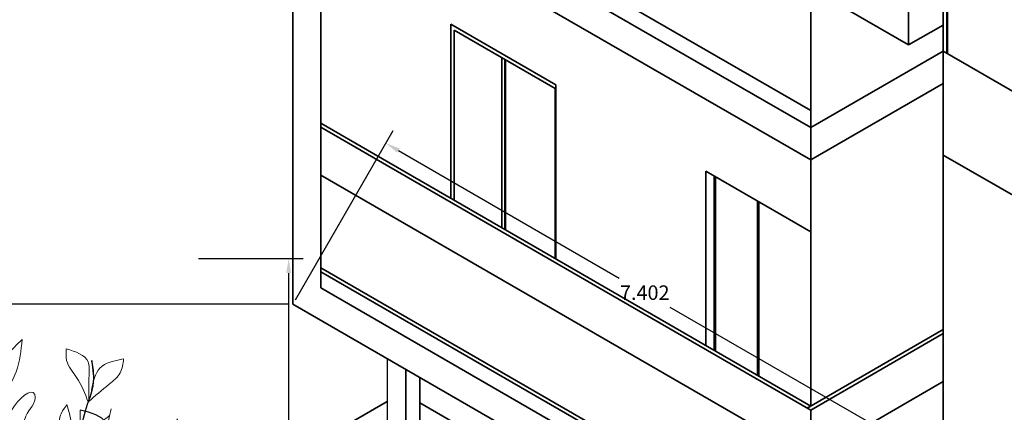
# Model space of a CAD drawing. Units: metres. Extents: x 12735 to 25554, y 20954 to 41989.
# Tile 7 of 15: x 12743.95 to 12756.13, y 20974.68 to 20979.54. Entities that reach past the tile are written whole.
import ezdxf

# ---------------------------------------------------------------- set-up
doc = ezdxf.new("R2010")
doc.units = ezdxf.units.M
doc.layers.get('Defpoints').update_dxf_attribs({"lineweight": 13})
for name, color, linetype, lineweight in [('A-ANNO-DIMS', 2, 'Continuous', 18), ('A-ELEV', 7, 'Continuous', 35), ('C-SITE', 8, 'Continuous', 25), ('TREES', 72, 'Continuous', 18)]:
    doc.layers.add(name, color=color, linetype=linetype, lineweight=lineweight)
doc.layers.add('STEM', color=32, linetype='Continuous')
doc.styles.get("Standard").update_dxf_attribs({"font": 'arial.ttf'})
doc.dimstyles.get("Standard").update_dxf_attribs({"dimtxt": 0.18, "dimasz": 0.18, "dimexe": 0.18, "dimexo": 0.0625, "dimgap": 0.09, "dimtad": 0, "dimtih": 1, "dimtoh": 1, "dimdec": 4, "dimzin": 0, "dimdsep": 46, "dimtxsty": 'Standard', "dimcen": 0.09, "dimadec": 0, "dimazin": 0, "dimtfac": 1, "dimtdec": 4, "dimtofl": 0, "dimtmove": 0, "dimatfit": 3, "dimfxl": 1, "dimtolj": 1, "dimtzin": 0, "dimarcsym": 0})

# ---------------------------------------------------------------- blocks, each defined once
blk = doc.blocks.new('TREES')
blk.add_line((12743.7, 20972.648), (12743.7, 20972.648))
at = {"layer": 'STEM'}
for points, knots in [([(12743.791, 20972.546), (12743.793, 20972.564), (12743.795, 20972.582), (12743.797, 20972.6), (12743.801, 20972.637), (12743.806, 20972.674), (12743.81, 20972.711), (12743.845, 20973.018), (12743.938, 20973.826), (12743.743, 20974.806), (12743.607, 20975.634), (12743.413, 20975.893), (12743.333, 20975.999)], [-0.164913, -0.164913, -0.164913, -0.164913, -0.110972, -0.110972, -0.110972, 0, 0, 0, 0.920963, 2.426088, 2.990404, 3.384799, 3.384799, 3.384799, 3.384799]), ([(12743.7, 20972.648), (12743.691, 20972.807), (12743.671, 20973.194), (12743.257, 20973.699), (12743.111, 20974.379), (12743.038, 20974.998), (12742.993, 20975.377), (12742.974, 20975.54)], [0, 0, 0, 0, 0.469346, 1.137622, 1.869488, 2.521439, 3.013071, 3.013071, 3.013071, 3.013071]), ([(12743.874, 20972.227), (12743.898, 20972.277), (12743.921, 20972.328), (12743.945, 20972.378), (12744.022, 20972.541), (12744.105, 20972.717), (12744.205, 20972.963), (12744.312, 20973.088), (12744.183, 20973.501), (12744.667, 20973.973), (12744.707, 20974.64), (12744.896, 20975.012), (12744.823, 20975.434), (12744.85, 20975.23), (12744.867, 20975.1)], [-0.166951, -0.166951, -0.166951, -0.166951, 0, 0, 0, 0.539768, 0.582066, 0.798222, 0.98781, 1.7696, 2.524754, 2.899414, 3.105113, 3.460848, 3.460848, 3.460848, 3.460848]), ([(12743.728, 20972.218), (12743.63, 20972.372), (12743.383, 20972.76), (12742.753, 20973.07), (12742.291, 20973.419), (12741.984, 20973.759), (12741.959, 20974.098), (12741.675, 20974.346), (12741.563, 20974.543), (12741.494, 20974.663)], [0, 0, 0, 0, 0.542161, 1.359078, 2.03444, 2.290187, 2.703676, 2.968549, 3.382864, 3.382864, 3.382864, 3.382864]), ([(12743.967, 20971.294), (12743.987, 20971.335), (12744.006, 20971.376), (12744.026, 20971.417), (12744.057, 20971.483), (12744.088, 20971.549), (12744.119, 20971.615), (12744.196, 20971.778), (12744.279, 20971.954), (12744.378, 20972.2), (12744.486, 20972.325), (12744.357, 20972.738), (12744.836, 20973.215), (12744.895, 20973.862), (12745.051, 20974.269), (12745.045, 20974.62), (12744.834, 20974.67), (12744.7, 20974.701)], [-0.355099, -0.355099, -0.355099, -0.355099, -0.218492, -0.218492, -0.218492, 0, 0, 0, 0.539768, 0.582066, 0.798222, 0.98781, 1.7696, 2.524754, 2.899414, 3.105113, 3.460848, 3.460848, 3.460848, 3.460848]), ([(12744.175, 20971.633), (12744.383, 20971.767), (12744.692, 20971.967), (12745.149, 20972.305), (12745.828, 20972.463), (12745.606, 20973.185), (12745.967, 20973.583), (12745.99, 20973.882), (12746.002, 20974.029)], [0, 0, 0, 0, 0.736164, 1.094646, 1.754618, 2.392389, 2.840214, 3.27091, 3.27091, 3.27091, 3.27091]), ([(12743.381, 20973.588), (12743.52, 20973.4), (12743.728, 20973.118), (12743.725, 20972.776), (12743.724, 20972.661), (12743.724, 20972.661), (12743.724, 20972.661), (12743.724, 20972.661), (12743.724, 20972.65), (12743.724, 20972.639), (12743.724, 20972.627)], [0, 0, 0, 0, 0.673099, 1.009429, 1.009429, 1.009429, 1.009429, 1.009429, 1.009429, 1.043412, 1.043412, 1.043412, 1.043412]), ([(12743.814, 20972.505), (12743.817, 20972.531), (12743.819, 20972.556), (12743.822, 20972.581), (12743.827, 20972.63), (12743.832, 20972.679), (12743.838, 20972.727), (12743.847, 20972.813), (12743.865, 20972.982), (12743.864, 20973.152), (12743.864, 20973.236)], [-0.2227932, -0.2227932, -0.2227932, -0.2227932, -0.1464713, -0.1464713, -0.1464713, 0, 0, 0, 0.2578951, 0.5103882, 0.5103882, 0.5103882, 0.5103882]), ([(12743.902, 20971.717), (12743.93, 20971.754), (12743.959, 20971.791), (12743.988, 20971.829), (12743.988, 20971.829), (12743.988, 20971.829), (12743.988, 20971.829), (12744.096, 20971.973), (12744.236, 20972.16), (12744.082, 20972.476), (12744.347, 20972.598), (12744.368, 20972.766), (12744.376, 20972.837)], [-0.129757, -0.129757, -0.129757, -0.129757, 0, 0, 0, 0, 0, 0, 0.485118, 0.62751, 0.913144, 1.120766, 1.120766, 1.120766, 1.120766]), ([(12744.111, 20968.725), (12743.967, 20969.837), (12743.799, 20971.142), (12743.712, 20972.453), (12743.7, 20972.648)], [0, 0, 0, 0, 3.359203, 3.944548, 3.944548, 3.944548, 3.944548]), ([(12744.332, 20968.825), (12744.189, 20969.936), (12743.871, 20971.161), (12743.872, 20972.51), (12743.7, 20972.648)], [0, 0, 0, 0, 3.359203, 3.972384, 3.972384, 3.972384, 3.972384]), ([(12743.597, 20972.418), (12743.533, 20972.41), (12743.292, 20972.379), (12742.889, 20972.351), (12742.364, 20972.241), (12741.803, 20972.489), (12741.157, 20972.302), (12740.698, 20972.258), (12740.474, 20972.237)], [0, 0, 0, 0, 0.193148, 0.727923, 1.218416, 1.762371, 2.471743, 3.152626, 3.152626, 3.152626, 3.152626]), ([(12743.181, 20972.372), (12743.296, 20972.37), (12743.441, 20972.368), (12743.583, 20972.39), (12743.613, 20972.395)], [0, 0, 0, 0, 0.3435042, 0.4329772, 0.4329772, 0.4329772, 0.4329772]), ([(12743.948, 20971.264), (12743.975, 20971.305), (12744.002, 20971.345), (12744.029, 20971.386), (12744.029, 20971.386), (12744.029, 20971.386), (12744.029, 20971.386), (12744.129, 20971.55), (12744.289, 20971.812), (12744.368, 20972.107), (12744.398, 20972.218)], [-0.148605, -0.148605, -0.148605, -0.148605, 0, 0, 0, 0, 0, 0, 0.572176, 0.914425, 0.914425, 0.914425, 0.914425]), ([(12743.901, 20971.729), (12743.929, 20971.768), (12743.958, 20971.808), (12743.986, 20971.847), (12743.986, 20971.847), (12743.986, 20971.847), (12743.986, 20971.847), (12744.02, 20971.892), (12744.062, 20971.951), (12744.099, 20972.014), (12744.107, 20972.028)], [-0.1467707, -0.1467707, -0.1467707, -0.1467707, 0, 0, 0, 0, 0, 0, 0.1684242, 0.2179474, 0.2179474, 0.2179474, 0.2179474]), ([(12743.81, 20971.258), (12743.646, 20971.316), (12743.283, 20971.443), (12742.486, 20971.453), (12741.888, 20971.61), (12741.494, 20971.714)], [0, 0, 0, 0, 0.519056, 1.146346, 2.366016, 2.366016, 2.366016, 2.366016])]:
    blk.add_open_spline(points, degree=3, knots=knots, dxfattribs=at)
blk.add_open_spline([(12744.644, 20971.941), (12744.672, 20971.961), (12744.701, 20971.98), (12744.73, 20972)], degree=3, dxfattribs=at)
at = {"layer": 'TREES'}
for points, knots in [([(12743.584, 20975.586), (12743.37, 20975.718), (12743.075, 20975.9), (12743.022, 20976.725), (12743.333, 20976.097), (12743.574, 20975.612)], [0, 0, 0, 0, 0.724771, 1.002271, 1.932196, 1.932196, 1.932196, 1.932196]), ([(12743.021, 20975.14), (12742.985, 20975.224), (12742.928, 20975.356), (12742.766, 20975.539), (12742.854, 20975.638), (12742.901, 20975.69)], [0, 0, 0, 0, 0.2845416, 0.4465287, 0.6279758, 0.6279758, 0.6279758, 0.6279758]), ([(12743.021, 20975.14), (12743.019, 20975.277), (12743.016, 20975.483), (12742.921, 20975.662), (12742.889, 20975.721)], [0, 0, 0, 0, 0.4023849, 0.6031293, 0.6031293, 0.6031293, 0.6031293]), ([(12743.718, 20974.979), (12743.671, 20975.164), (12743.598, 20975.454), (12743.323, 20975.534), (12743.223, 20975.563)], [0, 0, 0, 0, 0.519429, 0.8155501, 0.8155501, 0.8155501, 0.8155501]), ([(12743.223, 20975.563), (12743.266, 20975.448), (12743.36, 20975.195), (12743.592, 20975.055), (12743.718, 20974.979)], [0, 0, 0, 0, 0.3595778, 0.7860105, 0.7860105, 0.7860105, 0.7860105]), ([(12743.737, 20974.871), (12743.729, 20975.055), (12743.718, 20975.333), (12743.914, 20975.516), (12743.981, 20975.578)], [0, 0, 0, 0, 0.5134638, 0.7779111, 0.7779111, 0.7779111, 0.7779111]), ([(12743.737, 20974.871), (12743.801, 20974.971), (12743.939, 20975.186), (12743.966, 20975.441), (12743.981, 20975.578)], [0, 0, 0, 0, 0.351068, 0.7565079, 0.7565079, 0.7565079, 0.7565079]), ([(12741.648, 20974.411), (12741.519, 20974.547), (12741.281, 20974.798), (12741.642, 20974.995), (12741.673, 20975.511), (12741.684, 20975.149), (12741.787, 20975.033), (12741.768, 20974.824), (12741.781, 20974.575), (12741.641, 20974.411), (12741.569, 20974.326)], [0, 0, 0, 0, 0.446457, 0.821839, 1.096823, 1.294203, 1.491123, 1.594729, 1.894892, 2.216107, 2.216107, 2.216107, 2.216107]), ([(12743.031, 20975.058), (12743.048, 20975.139), (12743.077, 20975.281), (12743.184, 20975.377), (12743.231, 20975.418)], [0, 0, 0, 0, 0.2398723, 0.4207027, 0.4207027, 0.4207027, 0.4207027]), ([(12743.037, 20975.007), (12743.075, 20975.058), (12743.166, 20975.181), (12743.207, 20975.33), (12743.231, 20975.418)], [0, 0, 0, 0, 0.1895117, 0.457602, 0.457602, 0.457602, 0.457602]), ([(12744.796, 20974.806), (12744.757, 20974.909), (12744.688, 20975.088), (12744.514, 20975.28), (12744.523, 20975.414), (12744.526, 20975.464)], [0, 0, 0, 0, 0.3323117, 0.5782809, 0.7232611, 0.7232611, 0.7232611, 0.7232611]), ([(12744.805, 20974.813), (12744.804, 20974.918), (12744.803, 20975.076), (12744.822, 20975.37), (12744.643, 20975.427), (12744.526, 20975.464)], [0, 0, 0, 0, 0.3224266, 0.4885617, 0.8037384, 0.8037384, 0.8037384, 0.8037384]), ([(12743.07, 20974.733), (12742.98, 20974.863), (12742.848, 20975.053), (12742.433, 20975.446), (12742.649, 20974.915), (12742.651, 20974.573), (12742.961, 20974.576), (12743.034, 20974.678), (12743.071, 20974.73)], [0, 0, 0, 0, 0.54832, 0.799685, 1.166614, 1.565159, 1.742127, 1.925713, 1.925713, 1.925713, 1.925713]), ([(12744.796, 20974.806), (12744.882, 20974.878), (12745.017, 20974.992), (12745.211, 20975.15), (12745.228, 20975.277), (12745.236, 20975.337)], [0, 0, 0, 0, 0.3416822, 0.5370609, 0.7122352, 0.7122352, 0.7122352, 0.7122352]), ([(12744.839, 20974.951), (12744.859, 20975.055), (12744.903, 20975.272), (12745.122, 20975.315), (12745.236, 20975.337)], [0, 0, 0, 0, 0.2913456, 0.6064398, 0.6064398, 0.6064398, 0.6064398]), ([(12743.814, 20974.4), (12743.798, 20974.494), (12743.764, 20974.693), (12744.115, 20975.006), (12744.156, 20974.79), (12744.01, 20974.677), (12743.989, 20974.434), (12743.864, 20974.438), (12743.809, 20974.439)], [0, 0, 0, 0, 0.311146, 0.650746, 0.669061, 0.940573, 1.125337, 1.270427, 1.270427, 1.270427, 1.270427]), ([(12743.191, 20974.047), (12743.14, 20974.139), (12743.026, 20974.346), (12743.367, 20974.877), (12743.354, 20974.597), (12743.309, 20974.413), (12743.358, 20974.125), (12743.218, 20974.059), (12743.191, 20974.047)], [0, 0, 0, 0, 0.337622, 0.758697, 0.837919, 1.040495, 1.406258, 1.489574, 1.489574, 1.489574, 1.489574]), ([(12744.509, 20973.941), (12744.486, 20974.093), (12744.451, 20974.322), (12744.425, 20974.623), (12744.504, 20974.731), (12744.534, 20974.773)], [0, 0, 0, 0, 0.4681587, 0.7056034, 0.8580265, 0.8580265, 0.8580265, 0.8580265]), ([(12744.534, 20974.773), (12744.556, 20974.698), (12744.634, 20974.425), (12744.562, 20974.144), (12744.509, 20973.941)], [0, 0, 0, 0, 0.2327329, 0.8431329, 0.8431329, 0.8431329, 0.8431329]), ([(12742.028, 20973.754), (12742.003, 20973.912), (12741.953, 20974.218), (12742.174, 20974.414), (12742.283, 20974.81), (12742.258, 20974.48), (12742.304, 20974.323), (12742.246, 20974.069), (12742.227, 20973.932), (12742.006, 20973.671), (12742.066, 20973.72), (12742.075, 20973.727)], [0, 0, 0, 0, 0.436736, 0.842969, 1.012738, 1.21393, 1.403734, 1.613178, 1.897283, 2.067562, 2.097274, 2.097274, 2.097274, 2.097274]), ([(12744.554, 20973.975), (12744.669, 20974.016), (12744.893, 20974.094), (12745.019, 20974.421), (12745.06, 20974.624), (12745.08, 20974.72)], [0, 0, 0, 0, 0.348929, 0.678298, 0.9763146, 0.9763146, 0.9763146, 0.9763146]), ([(12744.97, 20974.043), (12744.931, 20974.146), (12744.862, 20974.325), (12744.688, 20974.517), (12744.697, 20974.651), (12744.7, 20974.701)], [0, 0, 0, 0, 0.3323117, 0.5782809, 0.7232611, 0.7232611, 0.7232611, 0.7232611]), ([(12743.835, 20974.249), (12743.789, 20974.346), (12743.724, 20974.484), (12743.556, 20974.594), (12743.468, 20974.601), (12743.424, 20974.604)], [0, 0, 0, 0, 0.3158223, 0.4463774, 0.5774617, 0.5774617, 0.5774617, 0.5774617]), ([(12743.424, 20974.604), (12743.442, 20974.527), (12743.487, 20974.324), (12743.715, 20974.191), (12743.841, 20974.206), (12743.841, 20974.206)], [0, 0, 0, 0, 0.2361186, 0.6165307, 0.6167763, 0.6167763, 0.6167763, 0.6167763]), ([(12744.618, 20974.118), (12744.717, 20974.268), (12744.844, 20974.462), (12745.022, 20974.606), (12745.062, 20974.638)], [0, 0, 0, 0, 0.5333846, 0.686651, 0.686651, 0.686651, 0.686651]), ([(12744.97, 20974.043), (12745.056, 20974.115), (12745.191, 20974.229), (12745.385, 20974.387), (12745.402, 20974.514), (12745.41, 20974.574)], [0, 0, 0, 0, 0.3416822, 0.5370609, 0.7122352, 0.7122352, 0.7122352, 0.7122352]), ([(12745.013, 20974.188), (12745.033, 20974.292), (12745.077, 20974.509), (12745.296, 20974.552), (12745.41, 20974.574)], [0, 0, 0, 0, 0.2913456, 0.6064398, 0.6064398, 0.6064398, 0.6064398]), ([(12745.957, 20973.706), (12745.908, 20973.835), (12745.798, 20974.123), (12745.864, 20974.427), (12745.9, 20974.594)], [0, 0, 0, 0, 0.4051126, 0.906838, 0.906838, 0.906838, 0.906838]), ([(12745.9, 20974.594), (12745.955, 20974.471), (12746.037, 20974.287), (12746.01, 20974.092), (12746.002, 20974.029)], [0, 0, 0, 0, 0.3943838, 0.5836156, 0.5836156, 0.5836156, 0.5836156]), ([(12743.128, 20974.182), (12743.019, 20974.275), (12742.841, 20974.427), (12742.65, 20974.313), (12742.577, 20974.27)], [0, 0, 0, 0, 0.3785086, 0.6144536, 0.6144536, 0.6144536, 0.6144536]), ([(12745.785, 20973.361), (12745.68, 20973.449), (12745.404, 20973.684), (12745.451, 20974.057), (12745.481, 20974.288)], [0, 0, 0, 0, 0.391493, 1.034106, 1.034106, 1.034106, 1.034106]), ([(12745.481, 20974.288), (12745.577, 20974.138), (12745.76, 20973.855), (12745.777, 20973.519), (12745.785, 20973.361)], [0, 0, 0, 0, 0.5245256, 0.9915723, 0.9915723, 0.9915723, 0.9915723]), ([(12741.943, 20974.016), (12741.835, 20974.13), (12741.594, 20974.382), (12741.272, 20973.991), (12740.687, 20974.27), (12741.289, 20973.836), (12741.63, 20973.742), (12741.878, 20973.799), (12742.016, 20973.831)], [0, 0, 0, 0, 0.397812, 0.88569, 1.156328, 1.66735, 1.991498, 2.394837, 2.394837, 2.394837, 2.394837]), ([(12742.577, 20974.27), (12742.635, 20974.174), (12742.755, 20973.977), (12743.187, 20974.003), (12743.173, 20974.131), (12743.172, 20974.137)], [0, 0, 0, 0, 0.3386751, 0.6999446, 0.7185805, 0.7185805, 0.7185805, 0.7185805]), ([(12743.879, 20973.555), (12743.816, 20973.752), (12743.731, 20974.021), (12743.982, 20974.067), (12744.068, 20974.224), (12744.006, 20973.984), (12744.093, 20973.824), (12743.961, 20973.709), (12743.879, 20973.638)], [0, 0, 0, 0, 0.469961, 0.638827, 0.705595, 0.853148, 1.022788, 1.296962, 1.296962, 1.296962, 1.296962]), ([(12744.356, 20973.647), (12744.309, 20973.708), (12744.202, 20973.846), (12744.245, 20974.018), (12744.268, 20974.113)], [0, 0, 0, 0, 0.2209277, 0.4981889, 0.4981889, 0.4981889, 0.4981889]), ([(12744.268, 20974.113), (12744.323, 20974.065), (12744.46, 20973.94), (12744.395, 20973.758), (12744.356, 20973.647)], [0, 0, 0, 0, 0.203616, 0.5174389, 0.5174389, 0.5174389, 0.5174389]), ([(12742.389, 20973.356), (12742.341, 20973.437), (12742.234, 20973.617), (12742.458, 20973.799), (12742.48, 20973.946), (12742.486, 20973.991)], [0, 0, 0, 0, 0.251735, 0.5591808, 0.6938707, 0.6938707, 0.6938707, 0.6938707]), ([(12742.486, 20973.991), (12742.542, 20973.959), (12742.68, 20973.88), (12742.598, 20973.572), (12742.464, 20973.433), (12742.389, 20973.356)], [0, 0, 0, 0, 0.1746142, 0.4385715, 0.7703441, 0.7703441, 0.7703441, 0.7703441]), ([(12743.381, 20973.588), (12743.369, 20973.67), (12743.344, 20973.833), (12743.453, 20973.958), (12743.508, 20974.02)], [0, 0, 0, 0, 0.2360196, 0.4713289, 0.4713289, 0.4713289, 0.4713289]), ([(12743.381, 20973.588), (12743.434, 20973.649), (12743.541, 20973.774), (12743.519, 20973.937), (12743.508, 20974.02)], [0, 0, 0, 0, 0.2309694, 0.4699481, 0.4699481, 0.4699481, 0.4699481]), ([(12744.683, 20973.178), (12744.66, 20973.33), (12744.625, 20973.559), (12744.599, 20973.86), (12744.677, 20973.968), (12744.708, 20974.01)], [0, 0, 0, 0, 0.4681587, 0.7056034, 0.8580265, 0.8580265, 0.8580265, 0.8580265]), ([(12744.708, 20974.01), (12744.73, 20973.935), (12744.807, 20973.662), (12744.735, 20973.381), (12744.683, 20973.178)], [0, 0, 0, 0, 0.2327329, 0.8431329, 0.8431329, 0.8431329, 0.8431329]), ([(12744.728, 20973.213), (12744.843, 20973.253), (12745.067, 20973.331), (12745.193, 20973.658), (12745.234, 20973.861), (12745.254, 20973.957)], [0, 0, 0, 0, 0.348929, 0.678298, 0.9763146, 0.9763146, 0.9763146, 0.9763146]), ([(12743.851, 20973.09), (12743.747, 20973.196), (12743.578, 20973.368), (12743.647, 20973.644), (12743.671, 20973.769), (12743.679, 20973.81)], [0, 0, 0, 0, 0.4076044, 0.6640272, 0.7921335, 0.7921335, 0.7921335, 0.7921335]), ([(12743.679, 20973.81), (12743.708, 20973.778), (12743.776, 20973.703), (12743.798, 20973.443), (12743.829, 20973.238), (12743.851, 20973.09)], [0, 0, 0, 0, 0.125659, 0.2981213, 0.7527794, 0.7527794, 0.7527794, 0.7527794]), ([(12744.792, 20973.355), (12744.891, 20973.505), (12745.018, 20973.699), (12745.196, 20973.843), (12745.236, 20973.876)], [0, 0, 0, 0, 0.5333846, 0.686651, 0.686651, 0.686651, 0.686651]), ([(12742.221, 20973.506), (12741.989, 20973.602), (12741.674, 20973.731), (12741.536, 20973.471), (12741.5, 20973.404)], [0, 0, 0, 0, 0.6060397, 0.8197481, 0.8197481, 0.8197481, 0.8197481]), ([(12743.364, 20973.617), (12743.288, 20973.661), (12743.124, 20973.754), (12742.939, 20973.715), (12742.84, 20973.694)], [0, 0, 0, 0, 0.2535199, 0.5460217, 0.5460217, 0.5460217, 0.5460217]), ([(12742.84, 20973.694), (12742.956, 20973.634), (12743.128, 20973.545), (12743.306, 20973.6), (12743.364, 20973.617)], [0, 0, 0, 0, 0.369417, 0.546183, 0.546183, 0.546183, 0.546183]), ([(12743.253, 20972.784), (12743.147, 20972.854), (12742.919, 20973.005), (12742.8, 20973.728), (12742.973, 20973.491), (12743.022, 20973.422)], [0, 0, 0, 0, 0.420416, 0.90702, 1.103207, 1.103207, 1.103207, 1.103207]), ([(12743.864, 20973.236), (12743.891, 20973.272), (12743.952, 20973.35), (12744.077, 20973.438), (12744.058, 20973.527), (12744.051, 20973.558)], [0, 0, 0, 0, 0.1377377, 0.3031534, 0.3935537, 0.3935537, 0.3935537, 0.3935537]), ([(12743.866, 20973.267), (12743.872, 20973.352), (12743.881, 20973.49), (12744.004, 20973.539), (12744.051, 20973.558)], [0, 0, 0, 0, 0.2295676, 0.3730638, 0.3730638, 0.3730638, 0.3730638]), ([(12744.268, 20973.425), (12744.32, 20973.505), (12744.424, 20973.666), (12744.615, 20973.662), (12744.711, 20973.66)], [0, 0, 0, 0, 0.2669279, 0.5349854, 0.5349854, 0.5349854, 0.5349854]), ([(12744.268, 20973.425), (12744.336, 20973.433), (12744.51, 20973.454), (12744.635, 20973.582), (12744.711, 20973.66)], [0, 0, 0, 0, 0.1990667, 0.5143408, 0.5143408, 0.5143408, 0.5143408]), ([(12741.493, 20973.429), (12741.634, 20973.396), (12741.906, 20973.333), (12742.16, 20973.449), (12742.283, 20973.505)], [0, 0, 0, 0, 0.420024, 0.8136231, 0.8136231, 0.8136231, 0.8136231]), ([(12743.022, 20973.422), (12743.059, 20973.426), (12743.334, 20973.456), (12743.256, 20972.956), (12743.349, 20972.723), (12743.36, 20972.696)], [0, 0, 0, 0, 0.1039343, 0.7792863, 0.8705393, 0.8705393, 0.8705393, 0.8705393]), ([(12745.697, 20972.996), (12745.547, 20972.999), (12745.238, 20973.004), (12745.268, 20973.314), (12745.283, 20973.473)], [0, 0, 0, 0, 0.3799868, 0.779071, 0.779071, 0.779071, 0.779071]), ([(12745.283, 20973.473), (12745.354, 20973.458), (12745.585, 20973.409), (12745.651, 20973.165), (12745.697, 20972.996)], [0, 0, 0, 0, 0.2074949, 0.6743984, 0.6743984, 0.6743984, 0.6743984]), ([(12743.621, 20973.151), (12743.561, 20973.233), (12743.473, 20973.354), (12743.333, 20973.334), (12743.288, 20973.327)], [0, 0, 0, 0, 0.2726158, 0.4022356, 0.4022356, 0.4022356, 0.4022356]), ([(12743.288, 20973.327), (12743.325, 20973.265), (12743.399, 20973.138), (12743.546, 20973.147), (12743.621, 20973.151)], [0, 0, 0, 0, 0.199886, 0.4070645, 0.4070645, 0.4070645, 0.4070645]), ([(12744.53, 20972.884), (12744.482, 20972.945), (12744.376, 20973.084), (12744.419, 20973.255), (12744.442, 20973.351)], [0, 0, 0, 0, 0.2209277, 0.4981889, 0.4981889, 0.4981889, 0.4981889]), ([(12744.442, 20973.351), (12744.496, 20973.302), (12744.634, 20973.177), (12744.569, 20972.995), (12744.53, 20972.884)], [0, 0, 0, 0, 0.203616, 0.5174389, 0.5174389, 0.5174389, 0.5174389]), ([(12741.595, 20972.406), (12741.523, 20972.496), (12741.318, 20972.752), (12741.336, 20973.087), (12741.348, 20973.304)], [0, 0, 0, 0, 0.3390919, 0.9589007, 0.9589007, 0.9589007, 0.9589007]), ([(12741.348, 20973.304), (12741.406, 20973.227), (12741.6, 20972.969), (12741.591, 20972.637), (12741.585, 20972.405)], [0, 0, 0, 0, 0.2865181, 0.9509807, 0.9509807, 0.9509807, 0.9509807]), ([(12745.697, 20972.996), (12745.724, 20973.08), (12745.77, 20973.226), (12745.915, 20973.262), (12745.976, 20973.277)], [0, 0, 0, 0, 0.2439478, 0.4222058, 0.4222058, 0.4222058, 0.4222058]), ([(12745.697, 20972.996), (12745.764, 20973.024), (12745.897, 20973.078), (12745.95, 20973.211), (12745.976, 20973.277)], [0, 0, 0, 0, 0.2073861, 0.4117039, 0.4117039, 0.4117039, 0.4117039]), ([(12743.669, 20972.977), (12743.606, 20973.025), (12743.504, 20973.102), (12743.398, 20973.043), (12743.358, 20973.021)], [0, 0, 0, 0, 0.2119595, 0.340544, 0.340544, 0.340544, 0.340544]), ([(12744.074, 20972.655), (12744.086, 20972.673), (12744.124, 20972.731), (12743.998, 20972.782), (12744.014, 20972.867), (12744.011, 20972.925), (12744.052, 20972.944), (12744.07, 20973.015), (12743.988, 20973.027), (12743.97, 20973.091), (12744.03, 20973.11), (12744.072, 20973.132), (12744.097, 20973.169), (12744.133, 20973.163), (12744.172, 20973.164), (12744.216, 20973.136), (12744.296, 20973.17), (12744.282, 20973.105), (12744.259, 20973.057), (12744.341, 20973.048), (12744.328, 20972.986), (12744.32, 20972.935), (12744.299, 20972.884), (12744.258, 20972.852), (12744.236, 20972.821), (12744.215, 20972.805), (12744.179, 20972.793), (12744.139, 20972.807), (12744.095, 20972.746), (12744.111, 20972.739), (12744.111, 20972.739)], [0, 0, 0, 0, 0.055886, 0.185472, 0.25227, 0.305988, 0.338368, 0.378405, 0.48523, 0.4997, 0.565031, 0.618654, 0.656012, 0.680602, 0.71942, 0.77395, 0.836088, 0.890088, 0.913694, 0.979696, 1.032481, 1.0683, 1.142133, 1.186825, 1.224162, 1.25438, 1.26551, 1.333296, 1.383591, 1.385324, 1.385324, 1.385324, 1.385324]), ([(12742.983, 20972.961), (12742.799, 20973.009), (12742.463, 20973.098), (12742.071, 20972.928), (12741.893, 20972.798), (12741.839, 20972.759)], [0, 0, 0, 0, 0.553894, 1.01265, 1.215779, 1.215779, 1.215779, 1.215779]), ([(12741.839, 20972.759), (12741.949, 20972.7), (12742.323, 20972.501), (12742.684, 20972.786), (12742.939, 20972.987)], [0, 0, 0, 0, 0.355589, 1.206871, 1.206871, 1.206871, 1.206871]), ([(12743.358, 20973.021), (12743.426, 20972.983), (12743.527, 20972.926), (12743.633, 20972.964), (12743.669, 20972.977)], [0, 0, 0, 0, 0.2166399, 0.3265492, 0.3265492, 0.3265492, 0.3265492]), ([(12741.358, 20972.366), (12741.291, 20972.434), (12741.162, 20972.564), (12740.909, 20972.646), (12740.492, 20972.989), (12740.719, 20972.381), (12740.905, 20972.253), (12741.437, 20972.382), (12741.361, 20972.366), (12741.358, 20972.366)], [0, 0, 0, 0, 0.274554, 0.529523, 0.902439, 1.220606, 1.740632, 1.953969, 1.962894, 1.962894, 1.962894, 1.962894]), ([(12742.858, 20972.779), (12743.034, 20972.81), (12743.375, 20972.87), (12743.295, 20972.539), (12743.257, 20972.379)], [0, 0, 0, 0, 0.4156133, 0.8046117, 0.8046117, 0.8046117, 0.8046117]), ([(12744.299, 20972.615), (12744.284, 20972.657), (12744.255, 20972.734), (12744.322, 20972.816), (12744.34, 20972.869), (12744.347, 20972.89)], [0, 0, 0, 0, 0.1248577, 0.2264879, 0.2926557, 0.2926557, 0.2926557, 0.2926557]), ([(12744.442, 20972.662), (12744.494, 20972.743), (12744.598, 20972.903), (12744.789, 20972.899), (12744.885, 20972.897)], [0, 0, 0, 0, 0.2669279, 0.5349854, 0.5349854, 0.5349854, 0.5349854]), ([(12744.442, 20972.662), (12744.51, 20972.671), (12744.684, 20972.691), (12744.809, 20972.819), (12744.885, 20972.897)], [0, 0, 0, 0, 0.1990667, 0.5143408, 0.5143408, 0.5143408, 0.5143408]), ([(12745.557, 20972.46), (12745.505, 20972.545), (12745.415, 20972.69), (12745.509, 20972.826), (12745.548, 20972.882)], [0, 0, 0, 0, 0.2672291, 0.4594629, 0.4594629, 0.4594629, 0.4594629]), ([(12745.548, 20972.882), (12745.623, 20972.785), (12745.735, 20972.639), (12745.619, 20972.519), (12745.581, 20972.479)], [0, 0, 0, 0, 0.3063433, 0.4579535, 0.4579535, 0.4579535, 0.4579535]), ([(12745.681, 20972.634), (12745.776, 20972.643), (12745.97, 20972.661), (12746.056, 20972.838), (12746.1, 20972.929)], [0, 0, 0, 0, 0.2646598, 0.5464061, 0.5464061, 0.5464061, 0.5464061]), ([(12745.691, 20972.679), (12745.723, 20972.743), (12745.803, 20972.904), (12745.989, 20972.919), (12746.1, 20972.929)], [0, 0, 0, 0, 0.2025395, 0.5100625, 0.5100625, 0.5100625, 0.5100625]), ([(12743.257, 20972.379), (12743.071, 20972.409), (12742.794, 20972.453), (12742.842, 20972.698), (12742.858, 20972.779)], [0, 0, 0, 0, 0.4478858, 0.6692237, 0.6692237, 0.6692237, 0.6692237]), ([(12744.14, 20972.455), (12744.129, 20972.498), (12744.112, 20972.571), (12744.173, 20972.643), (12744.195, 20972.684), (12744.204, 20972.7)], [0, 0, 0, 0, 0.124617, 0.2107396, 0.2658134, 0.2658134, 0.2658134, 0.2658134]), ([(12744.14, 20972.455), (12744.155, 20972.485), (12744.181, 20972.535), (12744.225, 20972.615), (12744.212, 20972.669), (12744.204, 20972.7)], [0, 0, 0, 0, 0.1037237, 0.1704768, 0.2630686, 0.2630686, 0.2630686, 0.2630686]), ([(12745.276, 20972.317), (12745.252, 20972.391), (12745.204, 20972.544), (12745.32, 20972.655), (12745.379, 20972.712)], [0, 0, 0, 0, 0.2148949, 0.4418034, 0.4418034, 0.4418034, 0.4418034]), ([(12745.276, 20972.317), (12745.329, 20972.378), (12745.429, 20972.493), (12745.395, 20972.642), (12745.379, 20972.712)], [0, 0, 0, 0, 0.2259484, 0.4304915, 0.4304915, 0.4304915, 0.4304915]), ([(12740.645, 20972.254), (12740.532, 20972.287), (12740.33, 20972.345), (12740.37, 20972.543), (12740.387, 20972.63)], [0, 0, 0, 0, 0.300298, 0.5327787, 0.5327787, 0.5327787, 0.5327787]), ([(12740.387, 20972.63), (12740.446, 20972.602), (12740.598, 20972.53), (12740.627, 20972.359), (12740.645, 20972.254)], [0, 0, 0, 0, 0.1847401, 0.4807235, 0.4807235, 0.4807235, 0.4807235]), ([(12742.916, 20972.343), (12742.772, 20972.452), (12742.448, 20972.697), (12742.076, 20972.511), (12741.869, 20972.407)], [0, 0, 0, 0, 0.501704, 1.133573, 1.133573, 1.133573, 1.133573]), ([(12744.192, 20972.515), (12744.244, 20972.502), (12744.335, 20972.479), (12744.372, 20972.56), (12744.387, 20972.593)], [0, 0, 0, 0, 0.1401829, 0.239855, 0.239855, 0.239855, 0.239855]), ([(12744.25, 20972.55), (12744.272, 20972.566), (12744.314, 20972.595), (12744.364, 20972.594), (12744.387, 20972.593)], [0, 0, 0, 0, 0.0790636, 0.1468534, 0.1468534, 0.1468534, 0.1468534]), ([(12744.137, 20972.378), (12744.147, 20972.414), (12744.168, 20972.49), (12744.249, 20972.485), (12744.292, 20972.483)], [0, 0, 0, 0, 0.0982704, 0.2114853, 0.2114853, 0.2114853, 0.2114853]), ([(12744.137, 20972.378), (12744.171, 20972.382), (12744.241, 20972.388), (12744.274, 20972.45), (12744.292, 20972.483)], [0, 0, 0, 0, 0.0955829, 0.1975677, 0.1975677, 0.1975677, 0.1975677]), ([(12744.868, 20972.097), (12744.937, 20972.148), (12745.072, 20972.246), (12745.072, 20972.413), (12745.073, 20972.494)], [0, 0, 0, 0, 0.2403434, 0.4714363, 0.4714363, 0.4714363, 0.4714363]), ([(12744.868, 20972.097), (12744.895, 20972.212), (12744.931, 20972.363), (12745.046, 20972.458), (12745.074, 20972.481)], [0, 0, 0, 0, 0.3374321, 0.4432568, 0.4432568, 0.4432568, 0.4432568]), ([(12745.582, 20972.481), (12745.667, 20972.516), (12745.814, 20972.576), (12745.958, 20972.516), (12746.019, 20972.491)], [0, 0, 0, 0, 0.2625898, 0.453199, 0.453199, 0.453199, 0.453199]), ([(12745.582, 20972.481), (12745.658, 20972.433), (12745.808, 20972.341), (12745.95, 20972.442), (12746.019, 20972.491)], [0, 0, 0, 0, 0.2451587, 0.4783488, 0.4783488, 0.4783488, 0.4783488]), ([(12741.223, 20971.823), (12741.319, 20971.881), (12741.571, 20972.033), (12741.755, 20972.264), (12741.869, 20972.407)], [0, 0, 0, 0, 0.3340001, 0.876507, 0.876507, 0.876507, 0.876507]), ([(12741.595, 20972.406), (12741.515, 20972.319), (12741.356, 20972.147), (12741.267, 20971.93), (12741.223, 20971.823)], [0, 0, 0, 0, 0.3521388, 0.6963584, 0.6963584, 0.6963584, 0.6963584]), ([(12743.181, 20972.372), (12743.094, 20972.305), (12742.907, 20972.162), (12742.991, 20971.938), (12743.035, 20971.819)], [0, 0, 0, 0, 0.2977969, 0.6372286, 0.6372286, 0.6372286, 0.6372286]), ([(12743.035, 20971.819), (12743.147, 20971.88), (12743.383, 20972.009), (12743.25, 20972.247), (12743.181, 20972.372)], [0, 0, 0, 0, 0.3275492, 0.688496, 0.688496, 0.688496, 0.688496]), ([(12744.145, 20972.348), (12744.132, 20972.384), (12744.105, 20972.455), (12744.032, 20972.434), (12743.996, 20972.423)], [0, 0, 0, 0, 0.098996, 0.196743, 0.196743, 0.196743, 0.196743]), ([(12743.996, 20972.423), (12744.027, 20972.377), (12744.069, 20972.315), (12744.13, 20972.341), (12744.146, 20972.347)], [0, 0, 0, 0, 0.1368513, 0.185287, 0.185287, 0.185287, 0.185287]), ([(12745.422, 20972.381), (12745.493, 20972.379), (12745.657, 20972.373), (12745.791, 20972.276), (12745.866, 20972.222)], [0, 0, 0, 0, 0.2087211, 0.4811791, 0.4811791, 0.4811791, 0.4811791]), ([(12745.422, 20972.381), (12745.521, 20972.247), (12745.661, 20972.058), (12745.82, 20972.185), (12745.866, 20972.222)], [0, 0, 0, 0, 0.3912381, 0.5526272, 0.5526272, 0.5526272, 0.5526272]), ([(12740.645, 20972.254), (12740.54, 20972.264), (12740.318, 20972.286), (12740.252, 20972.07), (12740.216, 20971.955)], [0, 0, 0, 0, 0.2808571, 0.5946199, 0.5946199, 0.5946199, 0.5946199]), ([(12740.216, 20971.955), (12740.344, 20971.984), (12740.536, 20972.026), (12740.618, 20972.197), (12740.645, 20972.254)], [0, 0, 0, 0, 0.3624795, 0.5464116, 0.5464116, 0.5464116, 0.5464116]), ([(12740.757, 20972.265), (12740.712, 20972.237), (12740.573, 20972.15), (12740.673, 20971.993), (12740.741, 20971.887)], [0, 0, 0, 0, 0.1417373, 0.4445248, 0.4445248, 0.4445248, 0.4445248]), ([(12740.741, 20971.887), (12740.783, 20971.937), (12740.878, 20972.054), (12740.801, 20972.189), (12740.757, 20972.265)], [0, 0, 0, 0, 0.1798963, 0.4162104, 0.4162104, 0.4162104, 0.4162104]), ([(12742.453, 20972.29), (12742.257, 20972.189), (12741.999, 20972.056), (12742.001, 20971.792), (12742.002, 20971.729)], [0, 0, 0, 0, 0.5792647, 0.7616052, 0.7616052, 0.7616052, 0.7616052]), ([(12742.002, 20971.729), (12742.108, 20971.788), (12742.333, 20971.914), (12742.411, 20972.161), (12742.453, 20972.29)], [0, 0, 0, 0, 0.3533474, 0.7448355, 0.7448355, 0.7448355, 0.7448355]), ([(12744.116, 20972.018), (12744.075, 20972.065), (12744.007, 20972.143), (12744.05, 20972.231), (12744.028, 20972.351), (12744.072, 20972.271), (12744.09, 20972.201), (12744.221, 20972.106), (12744.146, 20972.042), (12744.116, 20972.018)], [0, 0, 0, 0, 0.1633748, 0.2727914, 0.3326965, 0.376171, 0.4524353, 0.6040881, 0.701786, 0.701786, 0.701786, 0.701786]), ([(12744.746, 20972.012), (12744.742, 20972.047), (12744.733, 20972.118), (12744.771, 20972.218), (12744.826, 20972.252), (12744.849, 20972.268)], [0, 0, 0, 0, 0.1066556, 0.2131282, 0.2966333, 0.2966333, 0.2966333, 0.2966333]), ([(12744.746, 20972.012), (12744.773, 20972.045), (12744.822, 20972.105), (12744.891, 20972.268), (12744.848, 20972.268), (12744.847, 20972.268)], [0, 0, 0, 0, 0.1585708, 0.2833525, 0.285588, 0.285588, 0.285588, 0.285588]), ([(12745.053, 20972.215), (12745.111, 20972.233), (12745.273, 20972.284), (12745.353, 20972.117), (12745.405, 20972.009)], [0, 0, 0, 0, 0.1646898, 0.4645687, 0.4645687, 0.4645687, 0.4645687]), ([(12745.053, 20972.215), (12745.087, 20972.171), (12745.174, 20972.057), (12745.317, 20972.027), (12745.405, 20972.009)], [0, 0, 0, 0, 0.1638697, 0.4194041, 0.4194041, 0.4194041, 0.4194041]), ([(12742.652, 20971.471), (12742.63, 20971.58), (12742.585, 20971.809), (12742.714, 20972.005), (12742.781, 20972.107)], [0, 0, 0, 0, 0.3207709, 0.6721329, 0.6721329, 0.6721329, 0.6721329]), ([(12742.652, 20971.471), (12742.732, 20971.545), (12742.92, 20971.718), (12742.832, 20971.965), (12742.781, 20972.107)], [0, 0, 0, 0, 0.3028446, 0.7080533, 0.7080533, 0.7080533, 0.7080533]), ([(12744.455, 20971.815), (12744.445, 20971.868), (12744.427, 20971.97), (12744.523, 20972.088), (12744.564, 20972.169), (12744.585, 20972.208)], [0, 0, 0, 0, 0.1538132, 0.2966411, 0.4292928, 0.4292928, 0.4292928, 0.4292928]), ([(12744.455, 20971.815), (12744.544, 20971.891), (12744.679, 20972.008), (12744.609, 20972.157), (12744.585, 20972.208)], [0, 0, 0, 0, 0.3019229, 0.4589929, 0.4589929, 0.4589929, 0.4589929]), ([(12742.314, 20971.521), (12742.225, 20971.627), (12742.039, 20971.851), (12741.746, 20971.851), (12741.593, 20971.851)], [0, 0, 0, 0, 0.3968877, 0.8302181, 0.8302181, 0.8302181, 0.8302181]), ([(12741.593, 20971.851), (12741.666, 20971.793), (12741.821, 20971.668), (12742.447, 20971.471), (12742.312, 20971.521), (12742.311, 20971.521)], [0, 0, 0, 0, 0.3696351, 0.7965164, 0.7990281, 0.7990281, 0.7990281, 0.7990281]), ([(12743.566, 20971.341), (12743.514, 20971.414), (12743.424, 20971.54), (12743.418, 20971.749), (12743.449, 20971.857), (12743.463, 20971.904)], [0, 0, 0, 0, 0.2632417, 0.4527737, 0.6011812, 0.6011812, 0.6011812, 0.6011812]), ([(12743.463, 20971.904), (12743.567, 20971.861), (12743.772, 20971.775), (12743.623, 20971.516), (12743.587, 20971.385), (12743.574, 20971.338)], [0, 0, 0, 0, 0.2799093, 0.5517077, 0.7021324, 0.7021324, 0.7021324, 0.7021324]), ([(12744.561, 20971.885), (12744.589, 20971.902), (12744.651, 20971.938), (12744.742, 20971.883), (12744.801, 20971.859), (12744.827, 20971.849)], [0, 0, 0, 0, 0.0920276, 0.2010844, 0.2860976, 0.2860976, 0.2860976, 0.2860976]), ([(12744.561, 20971.885), (12744.599, 20971.871), (12744.674, 20971.844), (12744.795, 20971.792), (12744.822, 20971.84), (12744.827, 20971.849)], [0, 0, 0, 0, 0.1330667, 0.2587888, 0.2884885, 0.2884885, 0.2884885, 0.2884885]), ([(12743.304, 20971.408), (12743.247, 20971.446), (12743.157, 20971.505), (12743.12, 20971.647), (12743.123, 20971.722), (12743.125, 20971.759)], [0, 0, 0, 0, 0.196607, 0.3084716, 0.4203856, 0.4203856, 0.4203856, 0.4203856]), ([(12743.125, 20971.759), (12743.154, 20971.73), (12743.251, 20971.635), (12743.282, 20971.501), (12743.304, 20971.408)], [0, 0, 0, 0, 0.1222515, 0.400195, 0.400195, 0.400195, 0.400195]), ([(12742.056, 20971.092), (12742.207, 20971.066), (12742.53, 20971.009), (12742.604, 20971.335), (12742.644, 20971.51)], [0, 0, 0, 0, 0.3982442, 0.8534889, 0.8534889, 0.8534889, 0.8534889]), ([(12742.547, 20971.484), (12742.396, 20971.478), (12742.124, 20971.467), (12742.077, 20971.207), (12742.056, 20971.092)], [0, 0, 0, 0, 0.3960722, 0.7115037, 0.7115037, 0.7115037, 0.7115037]), ([(12742.918, 20971.429), (12742.811, 20971.373), (12742.636, 20971.282), (12742.7, 20971.111), (12742.725, 20971.045)], [0, 0, 0, 0, 0.3055467, 0.4944991, 0.4944991, 0.4944991, 0.4944991]), ([(12742.725, 20971.045), (12742.787, 20971.086), (12742.922, 20971.175), (12742.92, 20971.34), (12742.918, 20971.429)], [0, 0, 0, 0, 0.2088213, 0.4571427, 0.4571427, 0.4571427, 0.4571427]), ([(12743.381, 20971.391), (12743.311, 20971.354), (12743.137, 20971.26), (12743.15, 20971.056), (12743.158, 20970.935)], [0, 0, 0, 0, 0.2232821, 0.551466, 0.551466, 0.551466, 0.551466]), ([(12743.158, 20970.935), (12743.238, 20970.974), (12743.421, 20971.065), (12743.396, 20971.274), (12743.381, 20971.391)], [0, 0, 0, 0, 0.2445355, 0.5611675, 0.5611675, 0.5611675, 0.5611675]), ([(12743.743, 20971.282), (12743.611, 20971.245), (12743.396, 20971.185), (12743.421, 20970.978), (12743.431, 20970.898)], [0, 0, 0, 0, 0.3473993, 0.565418, 0.565418, 0.565418, 0.565418]), ([(12743.431, 20970.898), (12743.517, 20970.939), (12743.683, 20971.018), (12743.723, 20971.196), (12743.743, 20971.282)], [0, 0, 0, 0, 0.2699816, 0.5191769, 0.5191769, 0.5191769, 0.5191769])]:
    blk.add_open_spline(points, degree=3, knots=knots, dxfattribs=at)
blk.add_open_spline([(12744.347, 20972.89), (12744.357, 20972.872), (12744.367, 20972.854), (12744.376, 20972.837)], degree=3, dxfattribs=at)
blk = doc.blocks.new('*D5')
at = {"layer": 'A-ANNO-DIMS', "color": 0, "lineweight": -2, "transparency": 16777216}
for p, q in [((12746.163, 20976.581), (12747.458, 20976.581)), ((12747.278, 20976.401), (12747.278, 20972.835)), ((12747.278, 20968.905), (12747.278, 20972.471)), ((12746.163, 20968.725), (12747.458, 20968.725))]:
    blk.add_line(p, q, dxfattribs=at)
at = {"layer": 'A-ANNO-DIMS', "color": 0, "transparency": 16777216}
for points in [[(12747.248, 20976.401), (12747.308, 20976.401), (12747.278, 20976.581)], [(12747.248, 20968.905), (12747.308, 20968.905), (12747.278, 20968.725)]]:
    blk.add_solid(points, dxfattribs=at)
at = {"layer": 'Defpoints', "color": 0, "transparency": 16777216}
for p in [(12746.1, 20976.581), (12747.278, 20976.581), (12746.1, 20968.725)]:
    blk.add_point(p, dxfattribs=at)
at = {"layer": 'A-ANNO-DIMS', "color": 0, "transparency": 16777216, "insert": (12747.278, 20972.653), "char_height": 0.18, "attachment_point": 5}
blk.add_mtext('\\A1;TREE 8 TYP.', dxfattribs=at)
blk = doc.blocks.new('*D10')
at = {"layer": 'A-ANNO-DIMS', "color": 0, "lineweight": -2, "transparency": 16777216}
for p, q in [((12766.645, 20994.825), (12783.484, 20994.825)), ((12783.304, 20994.645), (12783.304, 20975.781)), ((12783.304, 20956.553), (12783.304, 20975.417)), ((12755.849, 20956.373), (12783.484, 20956.373))]:
    blk.add_line(p, q, dxfattribs=at)
at = {"layer": 'A-ANNO-DIMS', "color": 0, "transparency": 16777216}
for points in [[(12783.274, 20994.645), (12783.334, 20994.645), (12783.304, 20994.825)], [(12783.274, 20956.553), (12783.334, 20956.553), (12783.304, 20956.373)]]:
    blk.add_solid(points, dxfattribs=at)
at = {"layer": 'Defpoints', "color": 0, "transparency": 16777216}
for p in [(12766.582, 20994.825), (12783.304, 20994.825), (12755.787, 20956.373)]:
    blk.add_point(p, dxfattribs=at)
at = {"layer": 'A-ANNO-DIMS', "color": 0, "transparency": 16777216, "insert": (12783.304, 20975.599), "char_height": 0.18, "attachment_point": 5}
blk.add_mtext('\\A1;38.45', dxfattribs=at)
blk = doc.blocks.new('*D19')
at = {"layer": 'A-ANNO-DIMS', "color": 0, "lineweight": -2, "transparency": 16777216}
for p, q in [((12747.33, 20976.079), (12747.33, 20997.336)), ((12773.306, 20974.774), (12773.306, 20997.336)), ((12747.51, 20997.156), (12759.853, 20997.156)), ((12773.126, 20997.156), (12760.783, 20997.156))]:
    blk.add_line(p, q, dxfattribs=at)
at = {"layer": 'A-ANNO-DIMS', "color": 0, "transparency": 16777216}
for points in [[(12747.51, 20997.186), (12747.51, 20997.126), (12747.33, 20997.156)], [(12773.126, 20997.186), (12773.126, 20997.126), (12773.306, 20997.156)]]:
    blk.add_solid(points, dxfattribs=at)
at = {"layer": 'Defpoints', "color": 0, "transparency": 16777216}
for p in [(12773.306, 20997.156), (12747.33, 20976.016), (12773.306, 20974.711)]:
    blk.add_point(p, dxfattribs=at)
at = {"layer": 'A-ANNO-DIMS', "color": 0, "transparency": 16777216, "insert": (12760.318, 20997.156), "char_height": 0.18, "attachment_point": 5}
blk.add_mtext('\\A1;25.976', dxfattribs=at)
blk = doc.blocks.new('*D20')
at = {"layer": 'A-ANNO-DIMS', "color": 0, "lineweight": -2, "transparency": 16777216}
for p, q in [((12747.267, 20981.902), (12735.363, 20981.902)), ((12735.543, 20981.722), (12735.543, 20979.141)), ((12735.543, 20976.196), (12735.543, 20978.777)), ((12747.267, 20976.016), (12735.363, 20976.016))]:
    blk.add_line(p, q, dxfattribs=at)
at = {"layer": 'A-ANNO-DIMS', "color": 0, "transparency": 16777216}
for points in [[(12735.513, 20981.722), (12735.573, 20981.722), (12735.543, 20981.902)], [(12735.513, 20976.196), (12735.573, 20976.196), (12735.543, 20976.016)]]:
    blk.add_solid(points, dxfattribs=at)
at = {"layer": 'Defpoints', "color": 0, "transparency": 16777216}
for p in [(12747.33, 20981.902), (12735.543, 20976.016), (12747.33, 20976.016)]:
    blk.add_point(p, dxfattribs=at)
at = {"layer": 'A-ANNO-DIMS', "color": 0, "transparency": 16777216, "insert": (12735.543, 20978.959), "char_height": 0.18, "attachment_point": 5}
blk.add_mtext('\\A1;5.886', dxfattribs=at)
blk = doc.blocks.new('*D21')
at = {"layer": 'A-ANNO-DIMS', "color": 0, "lineweight": -2, "transparency": 16777216}
for p, q in [((12747.361, 20976.07), (12748.57, 20978.164)), ((12748.636, 20977.918), (12751.37, 20976.339)), ((12754.734, 20974.397), (12752, 20975.976)), ((12753.771, 20972.369), (12754.98, 20974.463))]:
    blk.add_line(p, q, dxfattribs=at)
at = {"layer": 'A-ANNO-DIMS', "color": 0, "transparency": 16777216}
for points in [[(12748.651, 20977.944), (12748.621, 20977.892), (12748.48, 20978.008)], [(12754.749, 20974.423), (12754.719, 20974.371), (12754.89, 20974.307)]]:
    blk.add_solid(points, dxfattribs=at)
at = {"layer": 'Defpoints', "color": 0, "transparency": 16777216}
for p in [(12747.33, 20976.016), (12754.89, 20974.307), (12753.74, 20972.315)]:
    blk.add_point(p, dxfattribs=at)
at = {"layer": 'A-ANNO-DIMS', "color": 0, "transparency": 16777216, "insert": (12751.685, 20976.158), "char_height": 0.18, "attachment_point": 5}
blk.add_mtext('\\A1;7.402', dxfattribs=at)

msp = doc.modelspace()

# ---------------------------------------------------------------- linework, layer by layer
at = {"layer": 'A-ELEV'}
for p, q in [((12754.951, 20986.429), (12754.951, 20979.2251)), ((12755.379, 20985.821), (12755.379, 20979.4722)), ((12753.7402, 20978.2012), (12747.3297, 20981.9023)), ((12747.3297, 20981.9023), (12747.3297, 20976.0163)), ((12747.7704, 20981.859), (12753.7402, 20978.4124)), ((12753.7402, 20977.8012), (12747.6761, 20981.3023)), ((12747.6761, 20981.3023), (12747.6761, 20976.2163)), ((12755.4237, 20979.1215), (12755.4237, 20981.2507)), ((12755.4323, 20979.1165), (12755.4323, 20981.2457)), ((12755.379, 20979.1473), (12755.379, 20980.6585)), ((12753.7402, 20978.2012), (12753.7402, 20979.7124)), ((12754.951, 20979.2251), (12754.1896, 20979.6647)), ((12749.2848, 20977.3264), (12749.2848, 20979.483)), ((12749.2848, 20979.483), (12750.5839, 20978.733)), ((12749.3281, 20977.3014), (12749.3281, 20979.408)), ((12749.3281, 20979.408), (12750.5752, 20978.688)), ((12754.951, 20979.2251), (12755.379, 20979.4722)), ((12749.917, 20979.068), (12749.917, 20976.9614)), ((12749.9517, 20979.048), (12749.9517, 20976.9414)), ((12749.9603, 20979.043), (12749.9603, 20976.9364)), ((12755.379, 20979.1473), (12753.7402, 20978.2012)), ((12760.2287, 20976.3473), (12755.379, 20979.1473)), ((12755.379, 20979.1473), (12755.379, 20973.2613)), ((12750.5752, 20978.688), (12750.5752, 20976.5814)), ((12750.5839, 20978.733), (12750.5839, 20976.5764)), ((12755.379, 20978.7473), (12753.7402, 20977.8012)), ((12753.7402, 20974.7541), (12753.7402, 20978.4124)), ((12748.3313, 20977.8769), (12747.6761, 20978.2552)), ((12748.3313, 20977.8269), (12747.6761, 20978.2052)), ((12753.7402, 20974.7541), (12748.3313, 20977.8769)), ((12753.7402, 20974.7041), (12748.3313, 20977.8269)), ((12757.8038, 20976.4613), (12755.379, 20977.8613)), ((12747.6761, 20977.6118), (12753.7402, 20974.1107)), ((12752.4406, 20975.5044), (12752.4406, 20977.661)), ((12752.4406, 20977.661), (12753.7402, 20976.9107)), ((12752.5445, 20975.4444), (12752.5445, 20977.601)), ((12752.5618, 20975.4344), (12752.5618, 20977.591)), ((12753.0814, 20977.291), (12753.0814, 20975.1344)), ((12753.0987, 20977.281), (12753.0987, 20975.1244)), ((12753.7402, 20972.9652), (12747.6761, 20976.4663)), ((12753.7402, 20972.9152), (12747.6761, 20976.4163)), ((12753.7402, 20972.7152), (12747.6761, 20976.2163)), ((12753.7402, 20972.3152), (12747.3297, 20976.0163)), ((12755.379, 20975.7003), (12753.6969, 20974.7291)), ((12755.379, 20975.6503), (12753.7402, 20974.7041)), ((12748.7281, 20975.2089), (12748.7281, 20972.6165)), ((12748.9013, 20975.1089), (12748.9013, 20972.7165)), ((12753.7402, 20974.1107), (12755.379, 20975.0569)), ((12748.4969, 20974.8107), (12744.1586, 20972.306)), ((12750.937, 20973.6198), (12748.9013, 20974.7951)), ((12753.7402, 20972.3152), (12753.7402, 20974.7041))]:
    msp.add_line(p, q, dxfattribs=at)
at = {"layer": 'C-SITE'}
msp.add_line((12748.4969, 20975.3424), (12748.4969, 20972.75), dxfattribs=at)

# ---------------------------------------------------------------- block references
at = {"layer": 'TREES'}
msp.add_blockref('TREES', (0, 0), dxfattribs=at)

# ---------------------------------------------------------------- dimensions: what is measured, and where the dimension line sits
at = {"layer": 'A-ANNO-DIMS'}
dim = msp.add_linear_dim(base=(12773.3057, 20997.1564), p1=(12747.3297, 20976.0163), p2=(12773.3057, 20974.7113), dimstyle='Standard', override={"dimdec": 3, "dimlfac": 1, "dimrnd": 0, "dimzin": 0, "dimdsep": 46, "dimlunit": 2}, dxfattribs=at)
dim.commit()
dim.dimension.update_dxf_attribs({"geometry": '*D19', "text_midpoint": (12760.3177, 20997.1564)})
for base, p1, p2, angle, override, picture, middle in [((12783.3041, 20994.8247), (12755.7869, 20956.3734), (12766.582, 20994.8247), 90, {"dimdec": 2, "dimlfac": 1, "dimrnd": 0, "dimzin": 0, "dimdsep": 46, "dimlunit": 2}, '*D10', (12783.3041, 20975.599)), ((12735.5426, 20976.0163), (12747.3297, 20981.9023), (12747.3297, 20976.0163), 90, {"dimdec": 3, "dimlfac": 1, "dimrnd": 0, "dimzin": 0, "dimdsep": 46, "dimlunit": 2}, '*D20', (12735.5426, 20978.9593)), ((12754.8902, 20974.307), (12747.3297, 20976.0163), (12753.7402, 20972.3152), 330, {"dimdec": 3, "dimlfac": 1, "dimrnd": 0, "dimzin": 0, "dimdsep": 46, "dimlunit": 2}, '*D21', (12751.6849, 20976.1576))]:
    dim = msp.add_linear_dim(base=base, p1=p1, p2=p2, angle=angle, dimstyle='Standard', override=override, dxfattribs=at)
    dim.commit()
    dim.dimension.update_dxf_attribs({"geometry": picture, "text_midpoint": middle})
dim = msp.add_linear_dim(base=(12747.2785, 20976.5808), p1=(12746.1001, 20968.7254), p2=(12746.1001, 20976.5808), angle=90, text='TREE <> TYP.', dimstyle='Standard', override={"dimdec": 0, "dimlfac": 1, "dimrnd": 0, "dimzin": 0, "dimdsep": 46, "dimlunit": 2}, dxfattribs=at)
dim.commit()
dim.dimension.update_dxf_attribs({"geometry": '*D5', "text_midpoint": (12747.2785, 20972.6531)})

doc.saveas('drawing.dxf')
